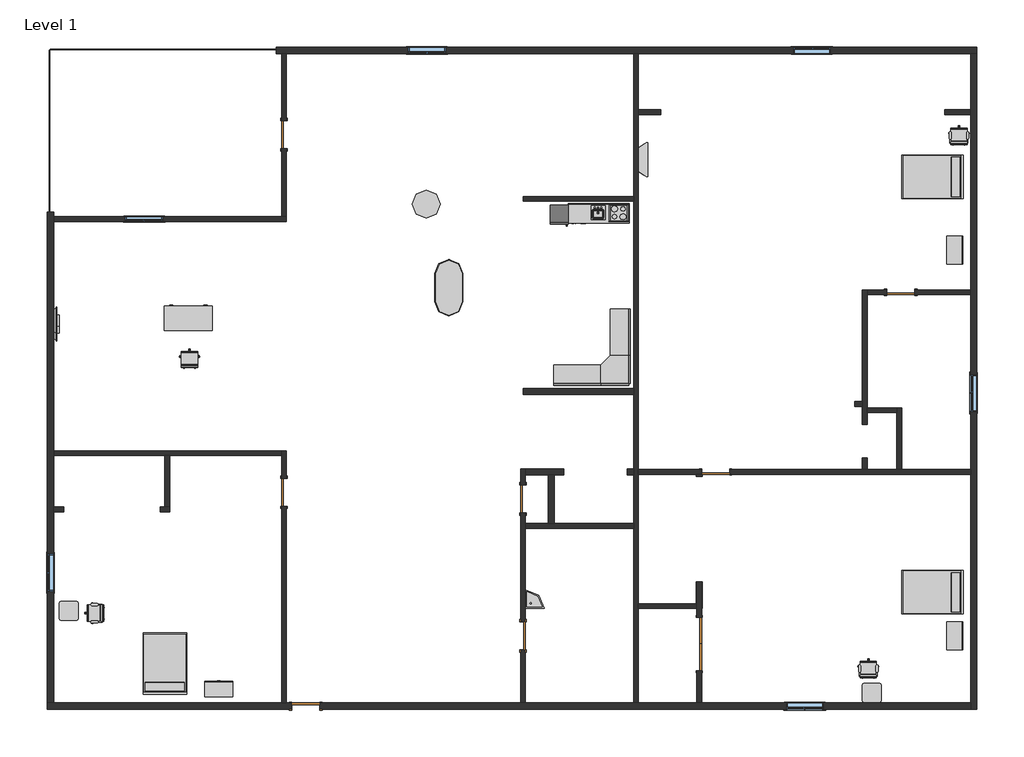
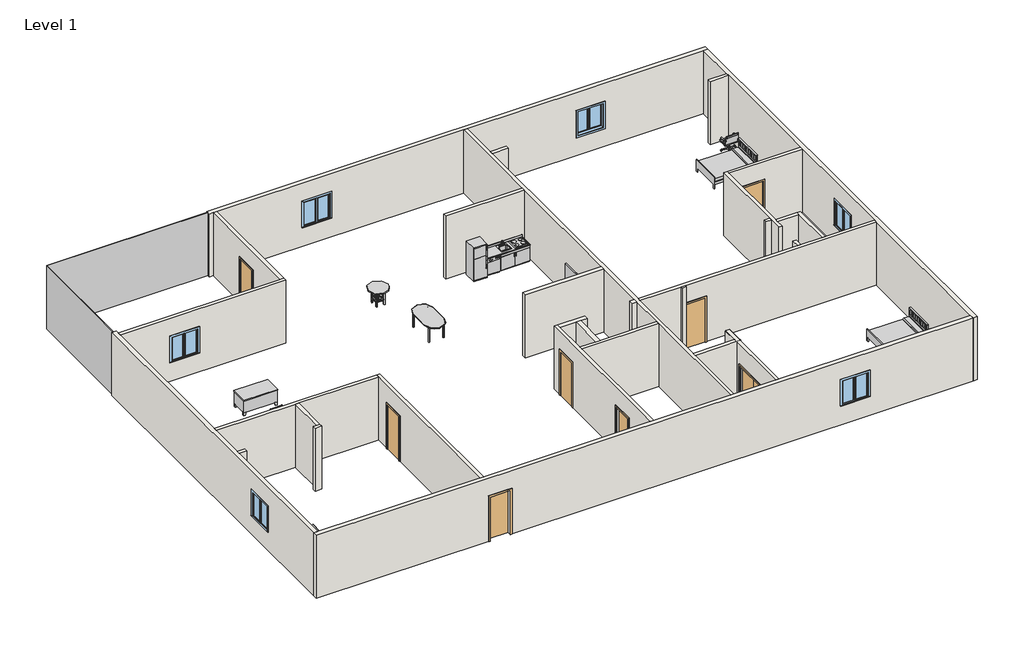
# One storey, incomplete: 32 walls, 20 furniture elements, 8 doors, 6 windows, 4 proxies, 2 flow terminals, 2 plates.
"""IFC4 building model written with IfcOpenShell, lengths in millimetres."""

from ifc_helpers import new_model, si_unit, frame, origin, origin_with_axes, place, context, project, spatial, polyline, outline, extrude, faceted_brep, transform, mapped, element, save
from components import proxy_dfcd9396, proxy_3c49123c, kitchenette_medium_kitchenette_medium_02f60b11, proxy_ec3341c2, door_74777eb6, door_54dd4da4, door_16372e1c, door_686f89d2, flow_terminal_bd5cdcf8, flow_terminal_41332a36, furniture_096e7f55, chair_task_chair_task_b7f3823b, chair_task_arms_chair_task_arms_fa5a08ef, furniture_dae9e1b9, furniture_072f6425, furniture_e1dba61b, furniture_56245f3a, tv_stand_tv_stand_6ce107e5, furniture_2c34a4f9, furniture_905aceb5, furniture_bcf351fa, furniture_45e3acac, system_panel_glazed_b550d99f, system_panel_glazed_2002d5d4, window_0862ab64, window_be30da88

model = new_model("IFC4")

# Units and contexts
model_context = context("Model", 3, world=origin())
ifc_project = project(units=[si_unit("LENGTHUNIT", "METRE", prefix="MILLI")], contexts=[model_context])

# Site, building, storey
site = spatial("IfcSite", under=ifc_project)
building = spatial("IfcBuilding", under=site)
storey = spatial("IfcBuildingStorey", under=building, Name="Level 1", Elevation=0.0)

# Proxies
placement = place(None, origin())
proxy_shape = proxy_dfcd9396(model_context)
element("IfcBuildingElementProxy", 1, Name="Cook Top-4 Unit2 : 22\" x 20\"", ObjectType="Cook Top-4 Unit2 : 22\" x 20\"", at=placement, inside=storey, context=model_context, shape_type="MappedRepresentation", body=[
    mapped(proxy_shape, transform((964.8533696, 8246.9729822, 0.0), x_axis=(-1.0, 0.0, 0.0), y_axis=(0.0, -1.0, 0.0), z_axis=(0.0, 0.0, 1.0))),
])
proxy_2_shape = proxy_3c49123c(model_context)
element("IfcBuildingElementProxy", 2, Name="Dishwasher : 24\" x 24\" x 34\"", ObjectType="Dishwasher : 24\" x 24\" x 34\"", at=placement, inside=storey, context=model_context, shape_type="MappedRepresentation", body=[
    mapped(proxy_2_shape, transform((13.670838, 7955.1234174, 0.0), x_axis=(-1.0, 0.0, 0.0), y_axis=(0.0, -1.0, 0.0), z_axis=(0.0, 0.0, 1.0))),
])
kitchenette_medium_kitchenette_medium_shape = kitchenette_medium_kitchenette_medium_02f60b11(model_context)
element("IfcBuildingElementProxy", 3, Name="Kitchenette - Medium : Kitchenette - Medium", ObjectType="Kitchenette - Medium : Kitchenette - Medium", at=placement, inside=storey, context=model_context, shape_type="MappedRepresentation", body=[
    mapped(kitchenette_medium_kitchenette_medium_shape, transform((640.6910745, 8551.7729822, 0.0), x_axis=(-1.0, 0.0, 0.0), y_axis=(0.0, -1.0, 0.0), z_axis=(0.0, 0.0, 1.0))),
])
proxy_3_shape = proxy_ec3341c2(model_context)
element("IfcBuildingElementProxy", 4, Name="Refrigerator : 24\" x 25\" LH", ObjectType="Refrigerator : 24\" x 25\" LH", at=placement, inside=storey, context=model_context, shape_type="MappedRepresentation", body=[
    mapped(proxy_3_shape, transform((-971.8966304, 8201.3240107, 0.0), x_axis=(-1.0, 0.0, 0.0), y_axis=(0.0, -1.0, 0.0), z_axis=(0.0, 0.0, 1.0))),
])

# Doors
door_shape = door_74777eb6(model_context)
element("IfcDoor", 5, ObjectType="Door-Double-Flush_Panel : 68\" x 80\"", at=placement, inside=storey, context=model_context, shape_type="MappedRepresentation", body=[
    mapped(door_shape, transform((3580.4287794, -5786.5270178, 0.0), x_axis=(0.0, -1.0, 0.0), y_axis=(1.0, 0.0, 0.0), z_axis=(0.0, 0.0, 1.0))),
])
door_2_shape = door_54dd4da4(model_context)
element("IfcDoor", 6, ObjectType="Single-Flush : 36\" x 84\"", at=placement, inside=storey, context=model_context, shape_type="MappedRepresentation", body=[
    mapped(door_2_shape, transform((-9208.4712206, -7805.8270178, 0.0), x_axis=(1.0, 0.0, 0.0), y_axis=(0.0, 1.0, 0.0), z_axis=(0.0, 0.0, 1.0))),
])
door_3_shape = door_16372e1c(model_context)
element("IfcDoor", 7, ObjectType="Single-Flush : 36\" x 84\"", at=placement, inside=storey, context=model_context, shape_type="MappedRepresentation", body=[
    mapped(door_3_shape, transform((-9919.6712206, -846.2270178, 0.0), x_axis=(0.0, 1.0, 0.0), y_axis=(-1.0, 0.0, 0.0), z_axis=(0.0, 0.0, 1.0))),
])
element("IfcDoor", 8, ObjectType="Single-Flush : 36\" x 84\"", at=placement, inside=storey, context=model_context, shape_type="MappedRepresentation", body=[
    mapped(door_3_shape, transform((4113.8287794, -185.8270178, 0.0), x_axis=(-1.0, 0.0, 0.0), y_axis=(0.0, -1.0, 0.0), z_axis=(0.0, 0.0, 1.0))),
])
element("IfcDoor", 9, ObjectType="Single-Flush : 36\" x 84\"", at=placement, inside=storey, context=model_context, shape_type="MappedRepresentation", body=[
    mapped(door_3_shape, transform((10133.6287794, 5656.1729822, 0.0), x_axis=(-1.0, 0.0, 0.0), y_axis=(0.0, -1.0, 0.0), z_axis=(0.0, 0.0, 1.0))),
])
element("IfcDoor", 10, ObjectType="Single-Flush : 36\" x 84\"", at=placement, inside=storey, context=model_context, shape_type="MappedRepresentation", body=[
    mapped(door_3_shape, transform((-2147.2712206, -5519.8270178, 0.0), x_axis=(0.0, -1.0, 0.0), y_axis=(1.0, 0.0, 0.0), z_axis=(0.0, 0.0, 1.0))),
])
element("IfcDoor", 11, ObjectType="Single-Flush : 36\" x 84\"", at=placement, inside=storey, context=model_context, shape_type="MappedRepresentation", body=[
    mapped(door_3_shape, transform((-2147.2712206, -1062.1270178, 0.0), x_axis=(0.0, 1.0, 0.0), y_axis=(-1.0, 0.0, 0.0), z_axis=(0.0, 0.0, 1.0))),
])
door_4_shape = door_686f89d2(model_context)
element("IfcDoor", 12, ObjectType="Single-Flush : 36\" x 84\"", at=placement, inside=storey, context=model_context, shape_type="MappedRepresentation", body=[
    mapped(door_4_shape, transform((-9919.6712206, 10786.9729822, 0.0), x_axis=(0.0, -1.0, 0.0), y_axis=(1.0, 0.0, 0.0), z_axis=(0.0, 0.0, 1.0))),
])

# Flow terminals
flow_terminal_shape = flow_terminal_bd5cdcf8(model_context)
element("IfcFlowTerminal", 13, ObjectType="Sink - Corner Floor : 24\"", at=placement, inside=storey, context=model_context, shape_type="MappedRepresentation", body=[
    mapped(flow_terminal_shape, transform((-2071.0712206, -4630.8270178, 0.0), x_axis=(1.0, 0.0, 0.0), y_axis=(0.0, 1.0, 0.0), z_axis=(0.0, 0.0, 1.0))),
])
flow_terminal_2_shape = flow_terminal_41332a36(model_context)
element("IfcFlowTerminal", 14, ObjectType="Sink Kitchen-Island : 18\" x 18\"", at=placement, inside=storey, context=model_context, shape_type="MappedRepresentation", body=[
    mapped(flow_terminal_2_shape, transform((307.4426101, 8244.6275811, -14.4), x_axis=(-1.0, 0.0, 0.0), y_axis=(0.0, -1.0, 0.0), z_axis=(0.0, 0.0, 1.0))),
])

# Furniture
furniture_shape = furniture_096e7f55(model_context)
element("IfcFurniture", 15, ObjectType="Bed-Shaker : Double 56\" x 78\"", at=placement, inside=storey, context=model_context, shape_type="MappedRepresentation", body=[
    mapped(furniture_shape, transform((12146.5787794, 9396.3229822, 0.0), x_axis=(0.0, -1.0000000000000437, 0.0), y_axis=(1.0000000000000437, 0.0, 0.0), z_axis=(0.0, 0.0, 1.0))),
])
element("IfcFurniture", 16, ObjectType="Bed-Shaker : Double 56\" x 78\"", at=placement, inside=storey, context=model_context, shape_type="MappedRepresentation", body=[
    mapped(furniture_shape, transform((12146.5787794, -4116.4770178, 0.0), x_axis=(0.0, -1.0, 0.0), y_axis=(1.0, 0.0, 0.0), z_axis=(0.0, 0.0, 1.0))),
])
element("IfcFurniture", 17, ObjectType="Bed-Shaker : Double 56\" x 78\"", at=placement, inside=storey, context=model_context, shape_type="MappedRepresentation", body=[
    mapped(furniture_shape, transform((-13812.2212206, -7399.4270178, 0.0), x_axis=(-1.0000000000000004, 0.0, 0.0), y_axis=(0.0, -1.0000000000000004, 0.0), z_axis=(0.0, 0.0, 1.0))),
])
chair_task_chair_task_shape = chair_task_chair_task_b7f3823b(model_context)
element("IfcFurniture", 18, ObjectType="Chair-Task : Chair-Task", at=placement, inside=storey, context=model_context, shape_type="MappedRepresentation", body=[
    mapped(chair_task_chair_task_shape, transform((-13134.0620403, 3452.8270806, 0.0), x_axis=(1.000000000000001, 0.0, 0.0), y_axis=(0.0, 1.000000000000001, 0.0), z_axis=(0.0, 0.0, 1.0))),
])
chair_task_arms_chair_task_arms_shape = chair_task_arms_chair_task_arms_fa5a08ef(model_context)
element("IfcFurniture", 19, ObjectType="Chair-Task Arms : Chair-Task Arms", at=placement, inside=storey, context=model_context, shape_type="MappedRepresentation", body=[
    mapped(chair_task_arms_chair_task_arms_shape, transform((8938.5379597, -6630.9729194, 0.0), x_axis=(1.0, 0.0, 0.0), y_axis=(0.0, 1.0, 0.0), z_axis=(0.0, 0.0, 1.0))),
])
element("IfcFurniture", 20, ObjectType="Chair-Task Arms : Chair-Task Arms", at=placement, inside=storey, context=model_context, shape_type="MappedRepresentation", body=[
    mapped(chair_task_arms_chair_task_arms_shape, transform((-16034.825319, -4924.2178374, 0.0), x_axis=(0.0, 1.000000000000001, 0.0), y_axis=(-1.000000000000001, 0.0, 0.0), z_axis=(0.0, 0.0, 1.0))),
])
element("IfcFurniture", 21, ObjectType="Chair-Task Arms : Chair-Task Arms", at=placement, inside=storey, context=model_context, shape_type="MappedRepresentation", body=[
    mapped(chair_task_arms_chair_task_arms_shape, transform((11884.9379597, 10717.2270806, 0.0), x_axis=(1.0, 0.0, 0.0), y_axis=(0.0, 1.0, 0.0), z_axis=(0.0, 0.0, 1.0))),
])
furniture_2_shape = furniture_dae9e1b9(model_context)
element("IfcFurniture", 22, ObjectType="Counter Top w Sink Hole : 24\" Depth", at=placement, inside=storey, context=model_context, shape_type="MappedRepresentation", body=[
    mapped(furniture_2_shape, transform((107.2910745, 8551.7729822, -14.4), x_axis=(-1.0, 0.0, 0.0), y_axis=(0.0, -1.0, 0.0), z_axis=(0.0, 0.0, 1.0))),
])
furniture_3_shape = furniture_072f6425(model_context)
element("IfcFurniture", 23, ObjectType="Desk : 60\" x 30\"", at=placement, inside=storey, context=model_context, shape_type="MappedRepresentation", body=[
    mapped(furniture_3_shape, transform((-13793.1712206, 4436.9729822, 0.0), x_axis=(1.0, 0.0, 0.0), y_axis=(0.0, 1.0, 0.0), z_axis=(0.0, 0.0, 1.0))),
])
furniture_4_shape = furniture_e1dba61b(model_context)
element("IfcFurniture", 24, ObjectType="Storage Pedestal : 20\" x 36\" x 36\"", at=placement, inside=storey, context=model_context, shape_type="MappedRepresentation", body=[
    mapped(furniture_4_shape, transform((10958.2604033, 7207.7954962, 0.0), x_axis=(0.0, 1.0000000000000002, 0.0), y_axis=(-1.0000000000000002, 0.0, 0.0), z_axis=(0.0, 0.0, 1.0))),
])
element("IfcFurniture", 25, ObjectType="Storage Pedestal : 20\" x 36\" x 36\"", at=placement, inside=storey, context=model_context, shape_type="MappedRepresentation", body=[
    mapped(furniture_4_shape, transform((10958.2604033, -5339.8045038, 0.0), x_axis=(0.0, 1.0000000000000002, 0.0), y_axis=(-1.0000000000000002, 0.0, 0.0), z_axis=(0.0, 0.0, 1.0))),
])
element("IfcFurniture", 26, ObjectType="Storage Pedestal : 20\" x 36\" x 36\"", at=placement, inside=storey, context=model_context, shape_type="MappedRepresentation", body=[
    mapped(furniture_4_shape, transform((-12220.5937345, -8181.3453938, 0.0), x_axis=(-1.0000000000000004, 0.0, 0.0), y_axis=(0.0, -1.0000000000000004, 0.0), z_axis=(0.0, 0.0, 1.0))),
])
furniture_5_shape = furniture_56245f3a(model_context)
element("IfcFurniture", 27, ObjectType="TV - Flat Screen : 32\"", at=placement, inside=storey, context=model_context, shape_type="MappedRepresentation", body=[
    mapped(furniture_5_shape, transform((-17379.532597, 4745.7174964, 0.0), x_axis=(0.0, 1.0000000000000002, 0.0), y_axis=(-1.0000000000000002, 0.0, 0.0), z_axis=(0.0, 0.0, 1.0))),
])
element("IfcFurniture", 28, ObjectType="TV - Flat Screen : 32\"", at=placement, inside=storey, context=model_context, shape_type="MappedRepresentation", body=[
    mapped(furniture_5_shape, transform((-17379.532597, 4517.1174964, 0.0), x_axis=(0.0, 1.0000000000000002, 0.0), y_axis=(-1.0000000000000002, 0.0, 0.0), z_axis=(0.0, 0.0, 1.0))),
])
tv_stand_tv_stand_shape = tv_stand_tv_stand_6ce107e5(model_context)
element("IfcFurniture", 29, ObjectType="TV Stand : TV Stand", at=placement, inside=storey, context=model_context, shape_type="MappedRepresentation", body=[
    mapped(tv_stand_tv_stand_shape, transform((1446.8287794, 9848.9849802, 0.0), x_axis=(0.0, 1.0000000000000002, 0.0), y_axis=(-1.0000000000000002, 0.0, 0.0), z_axis=(0.0, 0.0, 1.0))),
])
furniture_6_shape = furniture_2c34a4f9(model_context)
element("IfcFurniture", 30, ObjectType="Table-Dining Oval : 36\" x 72\"", at=placement, inside=storey, context=model_context, shape_type="MappedRepresentation", body=[
    mapped(furniture_6_shape, transform((-4202.17286, 5406.7533101, 0.0), x_axis=(0.0, -1.0000000000001008, 0.0), y_axis=(1.0000000000001008, 0.0, 0.0), z_axis=(0.0, 0.0, 1.0))),
])
furniture_7_shape = furniture_905aceb5(model_context)
element("IfcFurniture", 31, ObjectType="Table-Dining Round w Chairs : 36\" Diameter", at=placement, inside=storey, context=model_context, shape_type="MappedRepresentation", body=[
    mapped(furniture_7_shape, transform((-5400.5531878, 8711.2516707, 0.0), x_axis=(1.0000000000000622, 0.0, 0.0), y_axis=(0.0, 1.0000000000000622, 0.0), z_axis=(0.0, 0.0, 1.0))),
])
furniture_8_shape = furniture_bcf351fa(model_context)
element("IfcFurniture", 32, ObjectType="Table-End : 24\" x 24\"", at=placement, inside=storey, context=model_context, shape_type="MappedRepresentation", body=[
    mapped(furniture_8_shape, transform((-17225.9048509, -4859.4270178, 0.0), x_axis=(1.0, 0.0, 0.0), y_axis=(0.0, 1.0, 0.0), z_axis=(0.0, 0.0, 1.0))),
])
element("IfcFurniture", 33, ObjectType="Table-End : 24\" x 24\"", at=placement, inside=storey, context=model_context, shape_type="MappedRepresentation", body=[
    mapped(furniture_8_shape, transform((8885.2951491, -7526.4270178, 0.0), x_axis=(1.0, 0.0, 0.0), y_axis=(0.0, 1.0, 0.0), z_axis=(0.0, 0.0, 1.0))),
])
furniture_9_shape = furniture_45e3acac(model_context)
element("IfcFurniture", 34, ObjectType="Work Station Cubicle : 96\" x 96\"", at=placement, inside=storey, context=model_context, shape_type="MappedRepresentation", body=[
    mapped(furniture_9_shape, transform((1213.4970272, 2138.5499746, 0.0), x_axis=(-1.0000000000000002, 0.0, 0.0), y_axis=(0.0, -1.0000000000000002, 0.0), z_axis=(0.0, 0.0, 1.0))),
])

# Plates
system_panel_glazed_shape = system_panel_glazed_b550d99f(model_context)
element("IfcPlate", 35, ObjectType="System Panel : Glazed", at=placement, inside=storey, context=model_context, shape_type="MappedRepresentation", body=[
    mapped(system_panel_glazed_shape, transform((-13843.9712206, 13530.1729822, 0.0), x_axis=(1.0, 0.0, 0.0), y_axis=(0.0, 1.0, 0.0), z_axis=(0.0, 0.0, 1.0))),
])
system_panel_glazed_2_shape = system_panel_glazed_2002d5d4(model_context)
element("IfcPlate", 36, ObjectType="System Panel : Glazed", at=placement, inside=storey, context=model_context, shape_type="MappedRepresentation", body=[
    mapped(system_panel_glazed_2_shape, transform((-17514.2712206, 10901.2729822, 0.0), x_axis=(0.0, 1.0, 0.0), y_axis=(-1.0, 0.0, 0.0), z_axis=(0.0, 0.0, 1.0))),
])

# Walls
element("IfcWall", 37, ObjectType="Generic - 8\"", at=placement, inside=storey, context=model_context, shape_type="Brep", body=[
    faceted_brep([(12406.9287794, -7704.2270178, 0.0), (3656.6287794, -7704.2270178, 0.0), (3504.2287794, -7704.2270178, 0.0), (1599.2287794, -7704.2270178, 0.0), (1446.8287794, -7704.2270178, 0.0), (-2071.0712206, -7704.2270178, 0.0), (-2223.4712206, -7704.2270178, 0.0), (-8751.2712206, -7704.2270178, 0.0), (-8751.2712206, -7704.2270178, 2133.6), (-9665.6712206, -7704.2270178, 2133.6), (-9665.6712206, -7704.2270178, 0.0), (-9843.4712206, -7704.2270178, 0.0), (-9995.8712206, -7704.2270178, 0.0), (-17412.6712206, -7704.2270178, 0.0), (-17615.8712206, -7704.2270178, 0.0), (-17615.8712206, -7704.2270178, 3048.0), (-17412.6712206, -7704.2270178, 3048.0), (-9995.8712206, -7704.2270178, 3048.0), (-9843.4712206, -7704.2270178, 3048.0), (-2223.4712206, -7704.2270178, 3048.0), (-2071.0712206, -7704.2270178, 3048.0), (1446.8287794, -7704.2270178, 3048.0), (1599.2287794, -7704.2270178, 3048.0), (3504.2287794, -7704.2270178, 3048.0), (3656.6287794, -7704.2270178, 3048.0), (12406.9287794, -7704.2270178, 3048.0), (6406.1787794, -7704.2270178, 2133.6), (6406.1787794, -7704.2270178, 914.4), (7625.3787794, -7704.2270178, 914.4), (7625.3787794, -7704.2270178, 2133.6), (-8751.2712206, -7907.4270178, 2133.6), (-8751.2712206, -7907.4270178, 0.0), (12406.9287794, -7907.4270178, 0.0), (12406.9287794, -7907.4270178, 3048.0), (-17615.8712206, -7907.4270178, 3048.0), (-17615.8712206, -7907.4270178, 0.0), (-9665.6712206, -7907.4270178, 0.0), (-9665.6712206, -7907.4270178, 2133.6), (6406.1787794, -7907.4270178, 2133.6), (7625.3787794, -7907.4270178, 2133.6), (7625.3787794, -7907.4270178, 914.4), (6406.1787794, -7907.4270178, 914.4)], [[[0, 1, 2, 3, 4, 5, 6, 7, 8, 9, 10, 11, 12, 13, 14, 15, 16, 17, 18, 19, 20, 21, 22, 23, 24, 25], [26, 27, 28, 29]], [[30, 31, 32, 33, 34, 35, 36, 37], [38, 39, 40, 41]], [[36, 35, 14, 13, 12, 11, 10]], [[32, 31, 7, 6, 5, 4, 3, 2, 1, 0]], [[25, 24, 23, 22, 21, 20, 19, 18, 17, 16, 15, 34, 33]], [[15, 14, 35, 34]], [[8, 7, 31, 30]], [[9, 8, 30, 37]], [[10, 9, 37, 36]], [[0, 25, 33, 32]], [[27, 26, 38, 41]], [[28, 27, 41, 40]], [[29, 28, 40, 39]], [[26, 29, 39, 38]]]),
])
element("IfcWall", 38, ObjectType="Generic - 8\"", at=placement, inside=storey, context=model_context, shape_type="Brep", body=[
    faceted_brep([(-17412.6712206, -7704.2270178, 0.0), (-17412.6712206, -1481.2270178, 0.0), (-17412.6712206, -1328.8270178, 0.0), (-17412.6712206, 347.5729822, 0.0), (-17412.6712206, 499.9729822, 0.0), (-17412.6712206, 7967.5729822, 0.0), (-17412.6712206, 8119.9729822, 0.0), (-17412.6712206, 8272.3729822, 0.0), (-17412.6712206, 8272.3729822, 3048.0), (-17412.6712206, 8119.9729822, 3048.0), (-17412.6712206, 7967.5729822, 3048.0), (-17412.6712206, 499.9729822, 3048.0), (-17412.6712206, 347.5729822, 3048.0), (-17412.6712206, -1328.8270178, 3048.0), (-17412.6712206, -1481.2270178, 3048.0), (-17412.6712206, -7704.2270178, 3048.0), (-17412.6712206, -2852.8270178, 2133.6), (-17412.6712206, -2852.8270178, 914.4), (-17412.6712206, -4072.0270178, 914.4), (-17412.6712206, -4072.0270178, 2133.6), (-17615.8712206, -7704.2270178, 0.0), (-17615.8712206, -7704.2270178, 3048.0), (-17615.8712206, 8272.3729822, 3048.0), (-17615.8712206, 8272.3729822, 0.0), (-17615.8712206, -2852.8270178, 2133.6), (-17615.8712206, -4072.0270178, 2133.6), (-17615.8712206, -4072.0270178, 914.4), (-17615.8712206, -2852.8270178, 914.4)], [[[0, 1, 2, 3, 4, 5, 6, 7, 8, 9, 10, 11, 12, 13, 14, 15], [16, 17, 18, 19]], [[20, 21, 22, 23], [24, 25, 26, 27]], [[7, 6, 5, 4, 3, 2, 1, 0, 20, 23]], [[8, 7, 23, 22]], [[15, 14, 13, 12, 11, 10, 9, 8, 22, 21]], [[0, 15, 21, 20]], [[17, 16, 24, 27]], [[18, 17, 27, 26]], [[19, 18, 26, 25]], [[16, 19, 25, 24]]]),
])
element("IfcWall", 39, ObjectType="Generic - 8\"", at=placement, inside=storey, context=model_context, shape_type="Brep", body=[
    faceted_brep([(12406.9287794, 13428.5729822, 0.0), (12406.9287794, 11599.7729822, 0.0), (12406.9287794, 11447.3729822, 0.0), (12406.9287794, 5732.3729822, 0.0), (12406.9287794, 5579.9729822, 0.0), (12406.9287794, -109.6270178, 0.0), (12406.9287794, -262.0270178, 0.0), (12406.9287794, -7704.2270178, 0.0), (12406.9287794, -7907.4270178, 0.0), (12406.9287794, -7907.4270178, 3048.0), (12406.9287794, -7704.2270178, 3048.0), (12406.9287794, -262.0270178, 3048.0), (12406.9287794, -109.6270178, 3048.0), (12406.9287794, 5579.9729822, 3048.0), (12406.9287794, 5732.3729822, 3048.0), (12406.9287794, 11447.3729822, 3048.0), (12406.9287794, 11599.7729822, 3048.0), (12406.9287794, 13428.5729822, 3048.0), (12406.9287794, 2989.1729822, 2133.6), (12406.9287794, 1769.9729822, 2133.6), (12406.9287794, 1769.9729822, 914.4), (12406.9287794, 2989.1729822, 914.4), (12610.1287794, 13428.5729822, 0.0), (12610.1287794, 13428.5729822, 3048.0), (12610.1287794, -7907.4270178, 3048.0), (12610.1287794, -7907.4270178, 0.0), (12610.1287794, 2989.1729822, 2133.6), (12610.1287794, 2989.1729822, 914.4), (12610.1287794, 1769.9729822, 914.4), (12610.1287794, 1769.9729822, 2133.6)], [[[0, 1, 2, 3, 4, 5, 6, 7, 8, 9, 10, 11, 12, 13, 14, 15, 16, 17], [18, 19, 20, 21]], [[22, 23, 24, 25], [26, 27, 28, 29]], [[8, 7, 6, 5, 4, 3, 2, 1, 0, 22, 25]], [[17, 16, 15, 14, 13, 12, 11, 10, 9, 24, 23]], [[0, 17, 23, 22]], [[9, 8, 25, 24]], [[27, 26, 18, 21]], [[28, 27, 21, 20]], [[29, 28, 20, 19]], [[26, 29, 19, 18]]]),
])
element("IfcWall", 40, ObjectType="Generic - 8\"", at=placement, inside=storey, context=model_context, shape_type="SweptSolid", body=[
    extrude(outline(polyline([(-2147.2712206, 2531.9729822), (1446.8287794, 2531.9729822), (1446.8287794, 2328.7729822), (-2147.2712206, 2328.7729822), (-2147.2712206, 2531.9729822)])), origin_with_axes(), (0.0, 0.0, 1.0), 3048.0),
])
element("IfcWall", 41, ObjectType="Generic - 8\"", at=placement, inside=storey, context=model_context, shape_type="Brep", body=[
    faceted_brep([(-2071.0712206, -287.4270178, 0.0), (-1334.4712206, -287.4270178, 0.0), (-1131.2712206, -287.4270178, 0.0), (-826.4712206, -287.4270178, 0.0), (-826.4712206, -287.4270178, 3048.0), (-1131.2712206, -287.4270178, 3048.0), (-1334.4712206, -287.4270178, 3048.0), (-2071.0712206, -287.4270178, 3048.0), (-2071.0712206, -84.2270178, 0.0), (-2071.0712206, -84.2270178, 3048.0), (-826.4712206, -84.2270178, 3048.0), (-826.4712206, -84.2270178, 0.0)], [[[0, 1, 2, 3, 4, 5, 6, 7]], [[8, 9, 10, 11]], [[3, 2, 1, 0, 8, 11]], [[4, 3, 11, 10]], [[7, 6, 5, 4, 10, 9]], [[0, 7, 9, 8]]]),
])
element("IfcWall", 42, ObjectType="Generic - 8\"", at=placement, inside=storey, context=model_context, shape_type="SweptSolid", body=[
    extrude(outline(polyline([(-1334.4712206, -1862.2270178), (-1334.4712206, -287.4270178), (-1131.2712206, -287.4270178), (-1131.2712206, -1862.2270178), (-1334.4712206, -1862.2270178)])), origin_with_axes(), (0.0, 0.0, 1.0), 3048.0),
])
element("IfcWall", 43, ObjectType="Generic - 8\"", at=placement, inside=storey, context=model_context, shape_type="SweptSolid", body=[
    extrude(outline(polyline([(1446.8287794, -287.4270178), (1243.6287794, -287.4270178), (1243.6287794, -84.2270178), (1446.8287794, -84.2270178), (1446.8287794, -287.4270178)])), origin_with_axes(), (0.0, 0.0, 1.0), 3048.0),
])
element("IfcWall", 44, ObjectType="Generic - 8\"", at=placement, inside=storey, context=model_context, shape_type="Brep", body=[
    faceted_brep([(3478.8287794, -262.0270178, 0.0), (3478.8287794, -338.2270178, 0.0), (3478.8287794, -338.2270178, 3048.0), (3478.8287794, -262.0270178, 3048.0), (3682.0287794, -262.0270178, 0.0), (3682.0287794, -262.0270178, 3048.0), (3682.0287794, -338.2270178, 3048.0), (3682.0287794, -338.2270178, 0.0), (3656.6287794, -262.0270178, 0.0)], [[[0, 1, 2, 3]], [[4, 5, 6, 7]], [[1, 0, 8, 4, 7]], [[2, 1, 7, 6]], [[3, 2, 6, 5]], [[0, 3, 5, 4, 8]]]),
])
element("IfcWall", 45, ObjectType="Generic - 8\"", at=placement, inside=storey, context=model_context, shape_type="SweptSolid", body=[
    extrude(outline(polyline([(3682.0287794, -3767.2270178), (3682.0287794, -4478.4270178), (3478.8287794, -4478.4270178), (3478.8287794, -3767.2270178), (3682.0287794, -3767.2270178)])), origin_with_axes(), (0.0, 0.0, 1.0), 3048.0),
])
element("IfcWall", 46, ObjectType="Generic - 8\"", at=placement, inside=storey, context=model_context, shape_type="Brep", body=[
    faceted_brep([(-10173.6712206, 13428.5729822, 0.0), (-9995.8712206, 13428.5729822, 0.0), (-9843.4712206, 13428.5729822, 0.0), (1446.8287794, 13428.5729822, 0.0), (1599.2287794, 13428.5729822, 0.0), (12406.9287794, 13428.5729822, 0.0), (12610.1287794, 13428.5729822, 0.0), (12610.1287794, 13428.5729822, 3048.0), (12406.9287794, 13428.5729822, 3048.0), (1599.2287794, 13428.5729822, 3048.0), (1446.8287794, 13428.5729822, 3048.0), (-9843.4712206, 13428.5729822, 3048.0), (-9995.8712206, 13428.5729822, 3048.0), (-10173.6712206, 13428.5729822, 3048.0), (-5881.0712206, 13428.5729822, 2133.6), (-4661.8712206, 13428.5729822, 2133.6), (-4661.8712206, 13428.5729822, 914.4), (-5881.0712206, 13428.5729822, 914.4), (7853.9787794, 13428.5729822, 2133.6), (7853.9787794, 13428.5729822, 914.4), (6634.7787794, 13428.5729822, 914.4), (6634.7787794, 13428.5729822, 2133.6), (-10173.6712206, 13631.7729822, 0.0), (-10173.6712206, 13631.7729822, 3048.0), (12610.1287794, 13631.7729822, 3048.0), (12610.1287794, 13631.7729822, 0.0), (-5881.0712206, 13631.7729822, 2133.6), (-5881.0712206, 13631.7729822, 914.4), (-4661.8712206, 13631.7729822, 914.4), (-4661.8712206, 13631.7729822, 2133.6), (7853.9787794, 13631.7729822, 2133.6), (6634.7787794, 13631.7729822, 2133.6), (6634.7787794, 13631.7729822, 914.4), (7853.9787794, 13631.7729822, 914.4)], [[[0, 1, 2, 3, 4, 5, 6, 7, 8, 9, 10, 11, 12, 13], [14, 15, 16, 17], [18, 19, 20, 21]], [[22, 23, 24, 25], [26, 27, 28, 29], [30, 31, 32, 33]], [[6, 5, 4, 3, 2, 1, 0, 22, 25]], [[13, 12, 11, 10, 9, 8, 7, 24, 23]], [[0, 13, 23, 22]], [[7, 6, 25, 24]], [[26, 29, 15, 14]], [[29, 28, 16, 15]], [[28, 27, 17, 16]], [[27, 26, 14, 17]], [[18, 21, 31, 30]], [[21, 20, 32, 31]], [[20, 19, 33, 32]], [[19, 18, 30, 33]]]),
])
element("IfcWall", 47, ObjectType="Generic inner wall 6\"", at=placement, inside=storey, context=model_context, shape_type="Brep", body=[
    faceted_brep([(-17412.6712206, 347.5729822, 0.0), (-13793.1712206, 347.5729822, 0.0), (-13640.7712206, 347.5729822, 0.0), (-9995.8712206, 347.5729822, 0.0), (-9995.8712206, 347.5729822, 3048.0), (-13640.7712206, 347.5729822, 3048.0), (-13793.1712206, 347.5729822, 3048.0), (-17412.6712206, 347.5729822, 3048.0), (-17412.6712206, 499.9729822, 0.0), (-17412.6712206, 499.9729822, 3048.0), (-9995.8712206, 499.9729822, 3048.0), (-9995.8712206, 499.9729822, 0.0)], [[[0, 1, 2, 3, 4, 5, 6, 7]], [[8, 9, 10, 11]], [[3, 2, 1, 0, 8, 11]], [[7, 6, 5, 4, 10, 9]], [[0, 7, 9, 8]], [[4, 3, 11, 10]]]),
])
element("IfcWall", 48, ObjectType="Generic inner wall 6\"", at=placement, inside=storey, context=model_context, shape_type="Brep", body=[
    faceted_brep([(-17412.6712206, 7967.5729822, 0.0), (-9843.4712206, 7967.5729822, 0.0), (-9843.4712206, 7967.5729822, 3048.0), (-17412.6712206, 7967.5729822, 3048.0), (-15075.8712206, 7967.5729822, 2133.6), (-13856.6712206, 7967.5729822, 2133.6), (-13856.6712206, 7967.5729822, 914.4), (-15075.8712206, 7967.5729822, 914.4), (-17412.6712206, 8119.9729822, 0.0), (-17412.6712206, 8119.9729822, 3048.0), (-9995.8712206, 8119.9729822, 3048.0), (-9843.4712206, 8119.9729822, 3048.0), (-9843.4712206, 8119.9729822, 0.0), (-9995.8712206, 8119.9729822, 0.0), (-15075.8712206, 8119.9729822, 2133.6), (-15075.8712206, 8119.9729822, 914.4), (-13856.6712206, 8119.9729822, 914.4), (-13856.6712206, 8119.9729822, 2133.6)], [[[0, 1, 2, 3], [4, 5, 6, 7]], [[8, 9, 10, 11, 12, 13], [14, 15, 16, 17]], [[1, 0, 8, 13, 12]], [[3, 2, 11, 10, 9]], [[0, 3, 9, 8]], [[15, 14, 4, 7]], [[16, 15, 7, 6]], [[17, 16, 6, 5]], [[14, 17, 5, 4]], [[2, 1, 12, 11]]]),
])
element("IfcWall", 49, ObjectType="Generic inner wall 6\"", at=placement, inside=storey, context=model_context, shape_type="Brep", body=[
    faceted_brep([(-9995.8712206, 499.9729822, 0.0), (-9995.8712206, 347.5729822, 0.0), (-9995.8712206, -389.0270178, 0.0), (-9995.8712206, -389.0270178, 2133.6), (-9995.8712206, -1303.4270178, 2133.6), (-9995.8712206, -1303.4270178, 0.0), (-9995.8712206, -7704.2270178, 0.0), (-9995.8712206, -7704.2270178, 3048.0), (-9995.8712206, 347.5729822, 3048.0), (-9995.8712206, 499.9729822, 3048.0), (-9843.4712206, -389.0270178, 2133.6), (-9843.4712206, -389.0270178, 0.0), (-9843.4712206, 499.9729822, 0.0), (-9843.4712206, 499.9729822, 3048.0), (-9843.4712206, -7704.2270178, 3048.0), (-9843.4712206, -7704.2270178, 0.0), (-9843.4712206, -1303.4270178, 0.0), (-9843.4712206, -1303.4270178, 2133.6)], [[[0, 1, 2, 3, 4, 5, 6, 7, 8, 9]], [[10, 11, 12, 13, 14, 15, 16, 17]], [[16, 15, 6, 5]], [[12, 11, 2, 1, 0]], [[9, 8, 7, 14, 13]], [[7, 6, 15, 14]], [[0, 9, 13, 12]], [[3, 2, 11, 10]], [[4, 3, 10, 17]], [[5, 4, 17, 16]]]),
])
element("IfcWall", 50, ObjectType="Generic inner wall 6\"", at=placement, inside=storey, context=model_context, shape_type="SweptSolid", body=[
    extrude(outline(polyline([(10329.7729822, 2133.6), (10329.7729822, 0.0), (8119.9729822, 0.0), (8119.9729822, 3048.0), (13428.5729822, 3048.0), (13428.5729822, 0.0), (11244.1729822, 0.0), (11244.1729822, 2133.6), (10329.7729822, 2133.6)])), frame((-9995.8712206, 0.0, 0.0), z_axis=(1.0, 0.0, 0.0), x_axis=(0.0, 1.0, 0.0)), (0.0, 0.0, 1.0), 152.4),
])
element("IfcWall", 51, ObjectType="Generic inner wall 6\"", at=placement, inside=storey, context=model_context, shape_type="SweptSolid", body=[
    extrude(outline(polyline([(-13793.1712206, -1328.8270178), (-13793.1712206, 347.5729822), (-13640.7712206, 347.5729822), (-13640.7712206, -1328.8270178), (-13793.1712206, -1328.8270178)])), origin_with_axes(), (0.0, 0.0, 1.0), 3048.0),
])
element("IfcWall", 52, ObjectType="Generic inner wall 6\"", at=placement, inside=storey, context=model_context, shape_type="Brep", body=[
    faceted_brep([(-13640.7712206, -1328.8270178, 0.0), (-13793.1712206, -1328.8270178, 0.0), (-13945.5712206, -1328.8270178, 0.0), (-13945.5712206, -1328.8270178, 3048.0), (-13793.1712206, -1328.8270178, 3048.0), (-13640.7712206, -1328.8270178, 3048.0), (-13640.7712206, -1481.2270178, 0.0), (-13640.7712206, -1481.2270178, 3048.0), (-13945.5712206, -1481.2270178, 3048.0), (-13945.5712206, -1481.2270178, 0.0)], [[[0, 1, 2, 3, 4, 5]], [[6, 7, 8, 9]], [[2, 1, 0, 6, 9]], [[3, 2, 9, 8]], [[5, 4, 3, 8, 7]], [[0, 5, 7, 6]]]),
])
element("IfcWall", 53, ObjectType="Generic inner wall 6\"", at=placement, inside=storey, context=model_context, shape_type="SweptSolid", body=[
    extrude(outline(polyline([(-17082.4712206, -1481.2270178), (-17412.6712206, -1481.2270178), (-17412.6712206, -1328.8270178), (-17082.4712206, -1328.8270178), (-17082.4712206, -1481.2270178)])), origin_with_axes(), (0.0, 0.0, 1.0), 3048.0),
])
element("IfcWall", 54, ObjectType="Generic inner wall 6\"", at=placement, inside=storey, context=model_context, shape_type="Brep", body=[
    faceted_brep([(-2071.0712206, -604.9270178, 2133.6), (-2071.0712206, -604.9270178, 0.0), (-2071.0712206, -287.4270178, 0.0), (-2071.0712206, -84.2270178, 0.0), (-2071.0712206, -84.2270178, 3048.0), (-2071.0712206, -287.4270178, 3048.0), (-2071.0712206, -1862.2270178, 3048.0), (-2071.0712206, -2014.6270178, 3048.0), (-2071.0712206, -7704.2270178, 3048.0), (-2071.0712206, -7704.2270178, 0.0), (-2071.0712206, -5977.0270178, 0.0), (-2071.0712206, -5977.0270178, 2133.6), (-2071.0712206, -5062.6270178, 2133.6), (-2071.0712206, -5062.6270178, 0.0), (-2071.0712206, -2014.6270178, 0.0), (-2071.0712206, -1862.2270178, 0.0), (-2071.0712206, -1519.3270178, 0.0), (-2071.0712206, -1519.3270178, 2133.6), (-2223.4712206, -84.2270178, 0.0), (-2223.4712206, -604.9270178, 0.0), (-2223.4712206, -604.9270178, 2133.6), (-2223.4712206, -1519.3270178, 2133.6), (-2223.4712206, -1519.3270178, 0.0), (-2223.4712206, -5062.6270178, 0.0), (-2223.4712206, -5062.6270178, 2133.6), (-2223.4712206, -5977.0270178, 2133.6), (-2223.4712206, -5977.0270178, 0.0), (-2223.4712206, -7704.2270178, 0.0), (-2223.4712206, -7704.2270178, 3048.0), (-2223.4712206, -84.2270178, 3048.0)], [[[0, 1, 2, 3, 4, 5, 6, 7, 8, 9, 10, 11, 12, 13, 14, 15, 16, 17]], [[18, 19, 20, 21, 22, 23, 24, 25, 26, 27, 28, 29]], [[27, 26, 10, 9]], [[3, 2, 1, 19, 18]], [[16, 15, 14, 13, 23, 22]], [[8, 7, 6, 5, 4, 29, 28]], [[9, 8, 28, 27]], [[11, 10, 26, 25]], [[12, 11, 25, 24]], [[13, 12, 24, 23]], [[20, 19, 1, 0]], [[21, 20, 0, 17]], [[22, 21, 17, 16]], [[4, 3, 18, 29]]]),
])
element("IfcWall", 55, ObjectType="Generic inner wall 6\"", at=placement, inside=storey, context=model_context, shape_type="Brep", body=[
    faceted_brep([(1446.8287794, 13428.5729822, 0.0), (1446.8287794, 8780.3729822, 0.0), (1446.8287794, 8627.9729822, 0.0), (1446.8287794, 2531.9729822, 0.0), (1446.8287794, 2328.7729822, 0.0), (1446.8287794, -84.2270178, 0.0), (1446.8287794, -287.4270178, 0.0), (1446.8287794, -1862.2270178, 0.0), (1446.8287794, -2014.6270178, 0.0), (1446.8287794, -7704.2270178, 0.0), (1446.8287794, -7704.2270178, 3048.0), (1446.8287794, -2014.6270178, 3048.0), (1446.8287794, -1862.2270178, 3048.0), (1446.8287794, -287.4270178, 3048.0), (1446.8287794, -84.2270178, 3048.0), (1446.8287794, 2328.7729822, 3048.0), (1446.8287794, 2531.9729822, 3048.0), (1446.8287794, 8627.9729822, 3048.0), (1446.8287794, 8780.3729822, 3048.0), (1446.8287794, 13428.5729822, 3048.0), (1599.2287794, 13428.5729822, 0.0), (1599.2287794, 13428.5729822, 3048.0), (1599.2287794, 11599.7729822, 3048.0), (1599.2287794, 11447.3729822, 3048.0), (1599.2287794, -109.6270178, 3048.0), (1599.2287794, -262.0270178, 3048.0), (1599.2287794, -4478.4270178, 3048.0), (1599.2287794, -4630.8270178, 3048.0), (1599.2287794, -7704.2270178, 3048.0), (1599.2287794, -7704.2270178, 0.0), (1599.2287794, -4630.8270178, 0.0), (1599.2287794, -4478.4270178, 0.0), (1599.2287794, -262.0270178, 0.0), (1599.2287794, -109.6270178, 0.0), (1599.2287794, 11447.3729822, 0.0), (1599.2287794, 11599.7729822, 0.0)], [[[0, 1, 2, 3, 4, 5, 6, 7, 8, 9, 10, 11, 12, 13, 14, 15, 16, 17, 18, 19]], [[20, 21, 22, 23, 24, 25, 26, 27, 28, 29, 30, 31, 32, 33, 34, 35]], [[9, 8, 7, 6, 5, 4, 3, 2, 1, 0, 20, 35, 34, 33, 32, 31, 30, 29]], [[19, 18, 17, 16, 15, 14, 13, 12, 11, 10, 28, 27, 26, 25, 24, 23, 22, 21]], [[10, 9, 29, 28]], [[0, 19, 21, 20]]]),
])
element("IfcWall", 56, ObjectType="Generic inner wall 6\"", at=placement, inside=storey, context=model_context, shape_type="SweptSolid", body=[
    extrude(outline(polyline([(2335.8287794, 11447.3729822), (1599.2287794, 11447.3729822), (1599.2287794, 11599.7729822), (2335.8287794, 11599.7729822), (2335.8287794, 11447.3729822)])), origin_with_axes(), (0.0, 0.0, 1.0), 3048.0),
])
element("IfcWall", 57, ObjectType="Generic inner wall 6\"", at=placement, inside=storey, context=model_context, shape_type="SweptSolid", body=[
    extrude(outline(polyline([(-2147.2712206, 8780.3729822), (1446.8287794, 8780.3729822), (1446.8287794, 8627.9729822), (-2147.2712206, 8627.9729822), (-2147.2712206, 8780.3729822)])), origin_with_axes(), (0.0, 0.0, 1.0), 3048.0),
])
element("IfcWall", 58, ObjectType="Generic inner wall 6\"", at=placement, inside=storey, context=model_context, shape_type="Brep", body=[
    faceted_brep([(1599.2287794, -262.0270178, 0.0), (3478.8287794, -262.0270178, 0.0), (3656.6287794, -262.0270178, 0.0), (3656.6287794, -262.0270178, 2133.6), (4571.0287794, -262.0270178, 2133.6), (4571.0287794, -262.0270178, 0.0), (12406.9287794, -262.0270178, 0.0), (12406.9287794, -262.0270178, 3048.0), (3682.0287794, -262.0270178, 3048.0), (3478.8287794, -262.0270178, 3048.0), (1599.2287794, -262.0270178, 3048.0), (3656.6287794, -109.6270178, 2133.6), (3656.6287794, -109.6270178, 0.0), (1599.2287794, -109.6270178, 0.0), (1599.2287794, -109.6270178, 3048.0), (8889.0287794, -109.6270178, 3048.0), (9041.4287794, -109.6270178, 3048.0), (10012.9787794, -109.6270178, 3048.0), (10165.3787794, -109.6270178, 3048.0), (12406.9287794, -109.6270178, 3048.0), (12406.9287794, -109.6270178, 0.0), (10165.3787794, -109.6270178, 0.0), (10012.9787794, -109.6270178, 0.0), (9041.4287794, -109.6270178, 0.0), (8889.0287794, -109.6270178, 0.0), (4571.0287794, -109.6270178, 0.0), (4571.0287794, -109.6270178, 2133.6)], [[[0, 1, 2, 3, 4, 5, 6, 7, 8, 9, 10]], [[11, 12, 13, 14, 15, 16, 17, 18, 19, 20, 21, 22, 23, 24, 25, 26]], [[13, 12, 2, 1, 0]], [[25, 24, 23, 22, 21, 20, 6, 5]], [[10, 9, 8, 7, 19, 18, 17, 16, 15, 14]], [[7, 6, 20, 19]], [[0, 10, 14, 13]], [[3, 2, 12, 11]], [[4, 3, 11, 26]], [[5, 4, 26, 25]]]),
])
element("IfcWall", 59, ObjectType="Generic inner wall 6\"", at=placement, inside=storey, context=model_context, shape_type="Brep", body=[
    faceted_brep([(10165.3787794, -109.6270178, 0.0), (10165.3787794, 1896.9729822, 0.0), (10165.3787794, 1896.9729822, 3048.0), (10165.3787794, -109.6270178, 3048.0), (10012.9787794, -109.6270178, 0.0), (10012.9787794, -109.6270178, 3048.0), (10012.9787794, 1744.5729822, 3048.0), (10012.9787794, 1896.9729822, 3048.0), (10012.9787794, 1896.9729822, 0.0), (10012.9787794, 1744.5729822, 0.0)], [[[0, 1, 2, 3]], [[4, 5, 6, 7, 8, 9]], [[1, 0, 4, 9, 8]], [[3, 2, 7, 6, 5]], [[0, 3, 5, 4]], [[2, 1, 8, 7]]]),
])
element("IfcWall", 60, ObjectType="Generic inner wall 6\"", at=placement, inside=storey, context=model_context, shape_type="Brep", body=[
    faceted_brep([(8889.0287794, 5732.3729822, 0.0), (8889.0287794, 2100.1729822, 0.0), (8889.0287794, 1947.7729822, 0.0), (8889.0287794, 1363.5729822, 0.0), (8889.0287794, 1363.5729822, 3048.0), (8889.0287794, 1947.7729822, 3048.0), (8889.0287794, 2100.1729822, 3048.0), (8889.0287794, 5732.3729822, 3048.0), (9041.4287794, 5732.3729822, 0.0), (9041.4287794, 5732.3729822, 3048.0), (9041.4287794, 5579.9729822, 3048.0), (9041.4287794, 1896.9729822, 3048.0), (9041.4287794, 1744.5729822, 3048.0), (9041.4287794, 1363.5729822, 3048.0), (9041.4287794, 1363.5729822, 0.0), (9041.4287794, 1744.5729822, 0.0), (9041.4287794, 1896.9729822, 0.0), (9041.4287794, 5579.9729822, 0.0)], [[[0, 1, 2, 3, 4, 5, 6, 7]], [[8, 9, 10, 11, 12, 13, 14, 15, 16, 17]], [[3, 2, 1, 0, 8, 17, 16, 15, 14]], [[4, 3, 14, 13]], [[7, 6, 5, 4, 13, 12, 11, 10, 9]], [[0, 7, 9, 8]]]),
])
element("IfcWall", 61, ObjectType="Generic inner wall 6\"", at=placement, inside=storey, context=model_context, shape_type="SweptSolid", body=[
    extrude(outline(polyline([(0.0, 9041.4287794), (0.0, 9676.4287794), (2133.6, 9676.4287794), (2133.6, 10590.8287794), (0.0, 10590.8287794), (0.0, 12406.9287794), (3048.0, 12406.9287794), (3048.0, 9041.4287794), (0.0, 9041.4287794)])), frame((0.0, 5579.9729822, 0.0), z_axis=(0.0, 1.0, 0.0), x_axis=(0.0, 0.0, 1.0)), (0.0, 0.0, 1.0), 152.4),
])
element("IfcWall", 62, ObjectType="Generic inner wall 6\"", at=placement, inside=storey, context=model_context, shape_type="SweptSolid", body=[
    extrude(outline(polyline([(11568.7287794, 11599.7729822), (12406.9287794, 11599.7729822), (12406.9287794, 11447.3729822), (11568.7287794, 11447.3729822), (11568.7287794, 11599.7729822)])), origin_with_axes(), (0.0, 0.0, 1.0), 3048.0),
])
element("IfcWall", 63, ObjectType="Generic inner wall 6\"", at=placement, inside=storey, context=model_context, shape_type="SweptSolid", body=[
    extrude(outline(polyline([(9041.4287794, 271.3729822), (9041.4287794, -109.6270178), (8889.0287794, -109.6270178), (8889.0287794, 271.3729822), (9041.4287794, 271.3729822)])), origin_with_axes(), (0.0, 0.0, 1.0), 3048.0),
])
element("IfcWall", 64, ObjectType="Generic inner wall 6\"", at=placement, inside=storey, context=model_context, shape_type="SweptSolid", body=[
    extrude(outline(polyline([(9041.4287794, 1896.9729822), (10012.9787794, 1896.9729822), (10012.9787794, 1744.5729822), (9041.4287794, 1744.5729822), (9041.4287794, 1896.9729822)])), origin_with_axes(), (0.0, 0.0, 1.0), 3048.0),
])
element("IfcWall", 65, ObjectType="Generic inner wall 6\"", at=placement, inside=storey, context=model_context, shape_type="SweptSolid", body=[
    extrude(outline(polyline([(8635.0287794, 2100.1729822), (8889.0287794, 2100.1729822), (8889.0287794, 1947.7729822), (8635.0287794, 1947.7729822), (8635.0287794, 2100.1729822)])), origin_with_axes(), (0.0, 0.0, 1.0), 3048.0),
])
element("IfcWall", 66, ObjectType="Generic inner wall 6\"", at=placement, inside=storey, context=model_context, shape_type="Brep", body=[
    faceted_brep([(-2071.0712206, -2014.6270178, 0.0), (1446.8287794, -2014.6270178, 0.0), (1446.8287794, -2014.6270178, 3048.0), (-2071.0712206, -2014.6270178, 3048.0), (-2071.0712206, -1862.2270178, 0.0), (-2071.0712206, -1862.2270178, 3048.0), (-1334.4712206, -1862.2270178, 3048.0), (-1131.2712206, -1862.2270178, 3048.0), (1446.8287794, -1862.2270178, 3048.0), (1446.8287794, -1862.2270178, 0.0), (-1131.2712206, -1862.2270178, 0.0), (-1334.4712206, -1862.2270178, 0.0)], [[[0, 1, 2, 3]], [[4, 5, 6, 7, 8, 9, 10, 11]], [[1, 0, 4, 11, 10, 9]], [[3, 2, 8, 7, 6, 5]], [[0, 3, 5, 4]], [[2, 1, 9, 8]]]),
])
element("IfcWall", 67, ObjectType="Generic inner wall 6\"", at=placement, inside=storey, context=model_context, shape_type="Brep", body=[
    faceted_brep([(1599.2287794, -4630.8270178, 0.0), (3682.0287794, -4630.8270178, 0.0), (3682.0287794, -4630.8270178, 3048.0), (1599.2287794, -4630.8270178, 3048.0), (1599.2287794, -4478.4270178, 0.0), (1599.2287794, -4478.4270178, 3048.0), (3478.8287794, -4478.4270178, 3048.0), (3682.0287794, -4478.4270178, 3048.0), (3682.0287794, -4478.4270178, 0.0), (3478.8287794, -4478.4270178, 0.0)], [[[0, 1, 2, 3]], [[4, 5, 6, 7, 8, 9]], [[1, 0, 4, 9, 8]], [[3, 2, 7, 6, 5]], [[0, 3, 5, 4]], [[2, 1, 8, 7]]]),
])
element("IfcWall", 68, ObjectType="Generic inner wall 6\"", at=placement, inside=storey, context=model_context, shape_type="SweptSolid", body=[
    extrude(outline(polyline([(-7704.2270178, 3048.0), (-3767.2270178, 3048.0), (-3767.2270178, 0.0), (-4922.9270178, 0.0), (-4922.9270178, 2032.0), (-6650.1270178, 2032.0), (-6650.1270178, 0.0), (-7704.2270178, 0.0), (-7704.2270178, 3048.0)])), frame((3504.2287794, 0.0, 0.0), z_axis=(1.0, 0.0, 0.0), x_axis=(0.0, 1.0, 0.0)), (0.0, 0.0, 1.0), 152.4),
])

# Windows
window_shape = window_0862ab64(model_context)
element("IfcWindow", 69, ObjectType="Casement Dbl with Trim : 48\" x 48\"", at=placement, inside=storey, context=model_context, shape_type="MappedRepresentation", body=[
    mapped(window_shape, transform((-5271.4712206, 13549.2229822, 0.0), x_axis=(-1.0, 0.0, 0.0), y_axis=(0.0, -1.0, 0.0), z_axis=(0.0, 0.0, 1.0))),
])
element("IfcWindow", 70, ObjectType="Casement Dbl with Trim : 48\" x 48\"", at=placement, inside=storey, context=model_context, shape_type="MappedRepresentation", body=[
    mapped(window_shape, transform((-17495.2212206, -3462.4270178, 0.0), x_axis=(0.0, 1.0, 0.0), y_axis=(-1.0, 0.0, 0.0), z_axis=(0.0, 0.0, 1.0))),
])
element("IfcWindow", 71, ObjectType="Casement Dbl with Trim : 48\" x 48\"", at=placement, inside=storey, context=model_context, shape_type="MappedRepresentation", body=[
    mapped(window_shape, transform((7244.3787794, 13511.1229822, 0.0), x_axis=(1.0, 0.0, 0.0), y_axis=(0.0, 1.0, 0.0), z_axis=(0.0, 0.0, 1.0))),
])
element("IfcWindow", 72, ObjectType="Casement Dbl with Trim : 48\" x 48\"", at=placement, inside=storey, context=model_context, shape_type="MappedRepresentation", body=[
    mapped(window_shape, transform((12527.5787794, 2379.5729822, 0.0), x_axis=(0.0, 1.0, 0.0), y_axis=(-1.0, 0.0, 0.0), z_axis=(0.0, 0.0, 1.0))),
])
element("IfcWindow", 73, ObjectType="Casement Dbl with Trim : 48\" x 48\"", at=placement, inside=storey, context=model_context, shape_type="MappedRepresentation", body=[
    mapped(window_shape, transform((7015.7787794, -7786.7770178, 0.0), x_axis=(-1.0, 0.0, 0.0), y_axis=(0.0, -1.0, 0.0), z_axis=(0.0, 0.0, 1.0))),
])
window_2_shape = window_be30da88(model_context)
element("IfcWindow", 74, ObjectType="Casement Dbl with Trim : 48\" x 48\"", at=placement, inside=storey, context=model_context, shape_type="MappedRepresentation", body=[
    mapped(window_2_shape, transform((-14466.2712206, 8062.8229822, 0.0), x_axis=(-1.0, 0.0, 0.0), y_axis=(0.0, -1.0, 0.0), z_axis=(0.0, 0.0, 1.0))),
])

save(model, "model.ifc")

# Revit data of these elements
# Type "Cook Top-4 Unit2 : 22\" x 20\""
#   Depth = 1' - 8"
#   Width = 1' - 10"
#   Burner Material = Steel, Chrome Plated
#   Cooktop Material = Steel, Polished
#   Default Elevation = 0
#   Assembly Code = ""
# Type "Dishwasher : 24\" x 24\" x 34\""
#   Label = "DW"
#   Assembly Code = "E1090400"
#   Depth = 2' - 0"
#   Height = 2' - 10"
#   Width = 2' - 0"
#   Dishwasher Material = Steel, Paint Finish, Ivory, Glossy
#   Panel Face Material = Plastic, Opaque Black
#   Default Elevation = 0
# Type "Kitchenette - Medium : Kitchenette - Medium"
#   Assembly Code = "E1090400"
#   Counter Length = 6' - 6"
#   Cabinet Width = 4' - 6"
#   Cabinet Height = 2' - 10 1/2"
#   Cabinet Depth = 2' - 0"
#   Toe Depth = 0' - 3"
#   Toe Height = 0' - 3 1/2"
#   Cabinet Material = Cabinets
#   Door/Drawer Material = Cabinets
#   Handle Material = Cabinets - Handles
#   Default Elevation = 0
# Type "Refrigerator : 24\" x 25\" LH"
#   Label = "REF."
#   Assembly Code = "E1090400"
#   Depth = 2' - 0 3/4"
#   Handle = 0' - 1 1/2"
#   Height = 5' - 3 1/2"
#   Rear Clearance = 0' - 2"
#   Top Door Height = 1' - 8"
#   Width = 1' - 11 1/2"
#   Material = Steel, Paint Finish, Ivory, Glossy
#   Default Elevation = 0
# Type "Door-Double-Flush_Panel : 68\" x 80\""
#   Type Mark = "8"
#   Construction Type Id = "DOOR"
#   Assembly Code = "C1020"
#   Analytic Construction = "Wooden"
#   Thickness = 0' - 2"
#   Thermal Resistance (R) = 2.5876 (h·ft²·°F)/BTU
#   Swing Angle [instance default] = 90.00°
#   Panel Width = 2' - 10"
#   Heat Transfer Coefficient (U) = 0.3865 BTU/(h·ft²·°F)
#   Height = 6' - 8"
#   Trim Projection Ext = 0' - 1"
#   Trim Projection Int = 0' - 1"
#   Trim Width = 0' - 3"
#   Width = 5' - 8"
#   Define Thermal Properties by = 1
#   Panel Material = Wood - Birch - Solid Stained Light Low Gloss
#   Trim Material = Paint - Sienna
#   Visual Light Transmittance = 0
#   Solar Heat Gain Coefficient = 0
#   Function = (empty or 0)
#   Wall Closure = (empty or 0)
# Type "Single-Flush : 36\" x 84\""
#   Type Mark = "1"
#   Construction Type Id = "MDOOR"
#   Assembly Code = "C1020"
#   Analytic Construction = "Metal"
#   Thickness = 0' - 2"
#   Heat Transfer Coefficient (U) = 0.651978 BTU/(h·ft²·°F)
#   Height = 7' - 0"
#   Trim Projection Ext = 0' - 1"
#   Trim Projection Int = 0' - 1"
#   Trim Width = 0' - 3"
#   Width = 3' - 0"
#   Define Thermal Properties by = 1
#   Door Material = Door - Panel
#   Frame Material = Door - Frame
#   Visual Light Transmittance = 0
#   Solar Heat Gain Coefficient = 0
#   Function = (empty or 0)
#   Wall Closure = (empty or 0)
# Type "Sink - Corner Floor : 24\""
#   WFU = 2
#   Sink Radius = 2' - 0"
#   Sink Depth = 0' - 3 1/2"
#   Sanitary Radius = 3/4"
#   Sanitary Diameter = 1 1/2"
#   Radius 1 = 1' - 10"
#   Edge Width = 0' - 2"
#   Sink Material = none
#   HWFU = 0
#   Default Elevation = 0
#   CWFU = 0
# Type "Sink Kitchen-Island : 18\" x 18\""
#   Assembly Code = "D2010410"
#   Counter Height = 3' - 0"
#   Depth = 1' - 6"
#   Width = 1' - 6"
#   Faucet Material = Steel, Polished
#   Sink Material = Steel, Polished
#   Default Elevation = 0
# Type "Bed-Shaker : Double 56\" x 78\""
#   Assembly Code = "E2020200"
#   Length = 6' - 6"
#   Width = 4' - 8"
#   Frame Material = Birch
#   Mattress Material = Linen, White
#   Default Elevation = 0
# Type "Chair-Task : Chair-Task"
#   Assembly Code = "E2020200"
#   Base Material = Plastic, Opaque Black
#   Caster Material = Plastic, Opaque Black
#   Seat/Back Material = Textile - Slate Blue
#   Default Elevation = 0
# Type "Chair-Task Arms : Chair-Task Arms"
#   Assembly Code = "E2020200"
#   Base Material = Plastic, Opaque Black
#   Caster Material = Plastic, Opaque Black
#   Seat/Back Material = Textile - Slate Blue
#   Default Elevation = 0
# Type "Counter Top w Sink Hole : 24\" Depth"
#   Assembly Code = "C1030400"
#   Counter Thickness = 0' - 1 1/2"
#   Depth = 2' - 1"
#   Height = 3' - 0"
#   Length [instance default] = 8' - 0"
#   Sink Location [instance default] = 2' - 0"
#   Sink Location To Wall [instance default] = 0' - 6"
#   Sink Opening Depth [instance default] = 1' - 3"
#   Sink Opening Width [instance default] = 2' - 3"
#   Counter Top Material = none
#   Default Elevation = 0
# Type "Desk : 60\" x 30\""
#   Assembly Code = "E2020200"
#   Depth = 2' - 6"
#   Height = 2' - 6"
#   Leg Height = 0' - 6"
#   Width = 5' - 0"
#   Body Material = Laminate, Ivory, Matte
#   Handle/Leg Material = Steel, Chrome Plated
#   Top Material = Cherry
#   Default Elevation = 0
# Type "Storage Pedestal : 20\" x 36\" x 36\""
#   Assembly Code = "E2020"
#   Depth = 1' - 8"
#   Height = 3' - 0"
#   Width = 3' - 0"
#   Cabinet Material = Steel, Paint Finish, Ivory, Glossy
#   Handles Material = Steel, Chrome Plated
#   Default Elevation = 0
# Type "TV - Flat Screen : 32\""
#   SinAng = 0' - 0.0193"
#   L = 2' - 3.79372"
#   H = 1' - 3.6354"
#   Thickness = 0' - 4.33071"
#   Diagonal = 2' - 7.88976"
#   CosAng = 0' - 0.03431"
#   Stand [instance default] = yes
#   Default Elevation = 0
# Type "TV Stand : TV Stand"
#   Depth = 1' - 6"
#   Width = 3' - 8"
#   Height = 1' - 7 1/2"
#   Finish = Melamine - Gray
#   Default Elevation = 0
# Type "Table-Dining Oval : 36\" x 72\""
#   Assembly Code = "E2020200"
#   Length = 6' - 0"
#   Width = 3' - 0"
#   Base Material = Steel, Chrome Plated
#   Top Material = Glass - Clear, Grey
#   Default Elevation = 0
#   Description = (empty or 0)
# Type "Table-Dining Round w Chairs : 36\" Diameter"
#   Assembly Code = "E2020200"
#   Radius = 1' - 6"
#   Diameter = 3' - 0"
#   Height = 2' - 6"
#   Chairs = 4
#   Base Material = Pine
#   Top Material = Laminate, Linen, Matte
#   Default Elevation = 0
# Type "Table-End : 24\" x 24\""
#   Assembly Code = "E2020200"
#   Height = 2' - 6"
#   Length = 2' - 0"
#   Width = 2' - 0"
#   Base Material = Birch
#   Top Material = Laminate, Ivory, Matte
#   Default Elevation = 0
# Type "Work Station Cubicle : 96\" x 96\""
#   Assembly Code = "E2020"
#   Desktop Height = 2' - 6"
#   Desktop1 Width = 2' - 0"
#   Desktop2 Width = 2' - 0"
#   Panel Height = 5' - 6"
#   Panel1 Length = 5' - 0"
#   Panel2 Length = 5' - 0"
#   Cube Panel Material = Textile - Light Gray
#   Work Top Material = Laminate, Ivory, Matte
#   Default Elevation = 0
# Type "System Panel : Glazed"
#   Construction Type Id = "GSP4R"
#   Analytic Construction = "1/8 in Pilkington single glazing"
#   Visual Light Transmittance = 0.9
#   Solar Heat Gain Coefficient = 0.86
#   Heat Transfer Coefficient (U) = 1.18115 BTU/(h·ft²·°F)
# Type "Generic - 8\""
#   Assembly Code = "B2010"
#   Layers, outside or top first: 0' - 8" no material (function 1)
# Type "Generic inner wall 6\""
#   Assembly Code = "B2010"
#   Layers, outside or top first: 0' - 6" no material (function 1)
# Type "Casement Dbl with Trim : 48\" x 48\""
#   Type Mark = "10"
#   Construction Type Id = "GSP4R"
#   Assembly Code = "B2020100"
#   Analytic Construction = "1/8 in Pilkington single glazing"
#   Visual Light Transmittance = 0.9
#   Solar Heat Gain Coefficient = 0.78
#   Heat Transfer Coefficient (U) = 0.6496 BTU/(h·ft²·°F)
#   Height = 4' - 0"
#   Default Sill Height = 3' - 0"
#   Trim Projection - Ext. = 0' - 0 1/2"
#   Trim Projection - Int. = 0' - 0 3/4"
#   Trim Width - Exterior = 0' - 3 1/2"
#   Trim Width - Interior = 0' - 3 1/2"
#   Width = 4' - 0"
#   Window Inset = 0' - 0 3/4"
#   Define Thermal Properties by = 1
#   Glass Pane Material = Glass
#   Sash Material = Sash
#   Trim Exterior Material = Trim
#   Trim Interior Material = Trim
#   Wall Closure = (empty or 0)
# Element 1 (IfcBuildingElementProxy, "Cook Top-4 Unit2 : 22\" x 20\"")
#   Phase Created = New Construction
#   Materials on its faces: "Steel, Chrome Plated", "Steel, Polished"
# Element 2 (IfcBuildingElementProxy, "Dishwasher : 24\" x 24\" x 34\"")
#   Phase Created = New Construction
#   Materials on its faces: "Steel, Paint Finish, Ivory, Glossy", "Plastic, Opaque Black"
# Element 3 (IfcBuildingElementProxy, "Kitchenette - Medium : Kitchenette - Medium")
#   Phase Created = New Construction
#   Materials on its faces: "Cabinets", "Cabinets - Handles"
# Element 4 (IfcBuildingElementProxy, "Refrigerator : 24\" x 25\" LH")
#   Phase Created = New Construction
#   Materials on its faces: "Steel, Paint Finish, Ivory, Glossy", "Steel, Chrome Plated"
# Element 5 (IfcDoor, "Door-Double-Flush_Panel : 68\" x 80\"")
#   Swing Angle = 90.00°
#   Phase Created = New Construction
#   Materials on its faces: "Paint - Sienna", "Wood - Birch - Solid Stained Light Low Gloss"
# Elements 6, 7, 8, 9, 10, 11, 12 (IfcDoor, "Single-Flush : 36\" x 84\"")
#   Phase Created = New Construction
#   Materials on its faces: "Door - Frame", "Door - Panel"
# Element 13 (IfcFlowTerminal, "Sink - Corner Floor : 24\"")
#   Mark = "2"
#   Phase Created = New Construction
# Element 14 (IfcFlowTerminal, "Sink Kitchen-Island : 18\" x 18\"")
#   Mark = "9"
#   Phase Created = New Construction
#   Materials on its faces: "Steel, Polished"
# Elements 15, 16, 17 (IfcFurniture, "Bed-Shaker : Double 56\" x 78\"")
#   Phase Created = New Construction
#   Materials on its faces: "Birch", "Linen, White"
# Element 18 (IfcFurniture, "Chair-Task : Chair-Task")
#   Phase Created = New Construction
#   Materials on its faces: "Plastic, Opaque Black", "Textile - Slate Blue"
# Elements 19, 20, 21 (IfcFurniture, "Chair-Task Arms : Chair-Task Arms")
#   Phase Created = New Construction
#   Materials on its faces: "Plastic, Opaque Black", "Textile - Slate Blue"
# Element 22 (IfcFurniture, "Counter Top w Sink Hole : 24\" Depth")
#   Sink Opening Depth = 1' - 2"
#   Sink Location To Wall = 0' - 6"
#   Length = 6' - 6"
#   Sink Location = 3' - 4"
#   Sink Opening Width = 1' - 4"
#   Phase Created = New Construction
#   Materials on its faces: "Counter Top"
# Element 23 (IfcFurniture, "Desk : 60\" x 30\"")
#   Phase Created = New Construction
#   Materials on its faces: "Steel, Chrome Plated", "Laminate, Ivory, Matte", "Cherry"
# Elements 24, 25, 26 (IfcFurniture, "Storage Pedestal : 20\" x 36\" x 36\"")
#   Phase Created = New Construction
#   Materials on its faces: "Steel, Paint Finish, Ivory, Glossy", "Steel, Chrome Plated"
# Elements 27, 28 (IfcFurniture, "TV - Flat Screen : 32\"")
#   Stand = yes
#   Phase Created = New Construction
#   Materials on its faces: "TV - Black", "TV - Glass", "TV - Screen"
